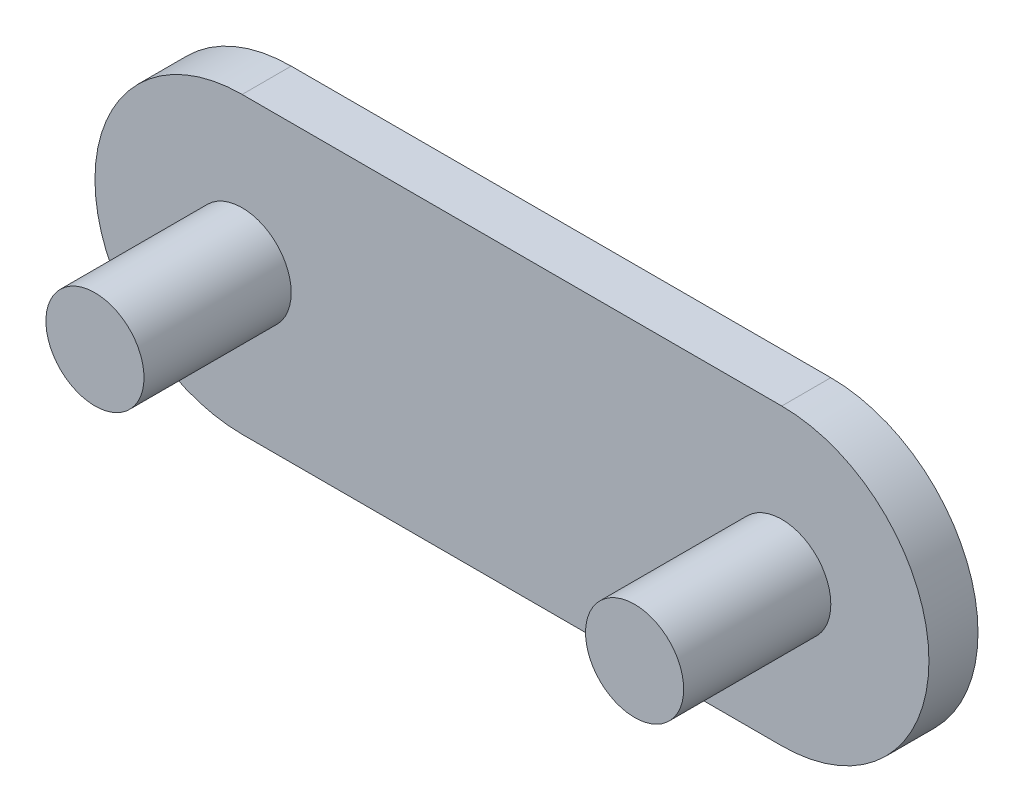
ISO-10303-21;
HEADER;
FILE_DESCRIPTION(('STEP AP214'),'2;1');
FILE_NAME('part.step','',(''),(''),'','','');
FILE_SCHEMA(('AUTOMOTIVE_DESIGN { 1 0 10303 214 1 1 1 1 }'));
ENDSEC;
DATA;
#1=APPLICATION_CONTEXT('core data for automotive mechanical design processes');
#2=APPLICATION_PROTOCOL_DEFINITION('international standard','automotive_design',2000,#1);
#3=PRODUCT_CONTEXT('',#1,'mechanical');
#4=PRODUCT('Part','Part','',(#3));
#5=PRODUCT_RELATED_PRODUCT_CATEGORY('part','',(#4));
#6=PRODUCT_DEFINITION_FORMATION('','',#4);
#7=PRODUCT_DEFINITION_CONTEXT('part definition',#1,'design');
#8=PRODUCT_DEFINITION('design','',#6,#7);
#9=PRODUCT_DEFINITION_SHAPE('','',#8);
#10=(LENGTH_UNIT() NAMED_UNIT(*) SI_UNIT(.MILLI.,.METRE.));
#11=(NAMED_UNIT(*) PLANE_ANGLE_UNIT() SI_UNIT($,.RADIAN.));
#12=(NAMED_UNIT(*) SI_UNIT($,.STERADIAN.) SOLID_ANGLE_UNIT());
#13=UNCERTAINTY_MEASURE_WITH_UNIT(LENGTH_MEASURE(1.E-05),#10,'distance_accuracy_value','');
#14=(GEOMETRIC_REPRESENTATION_CONTEXT(3) GLOBAL_UNCERTAINTY_ASSIGNED_CONTEXT((#13)) GLOBAL_UNIT_ASSIGNED_CONTEXT((#10,
#11,#12)) REPRESENTATION_CONTEXT('',''));
#15=CARTESIAN_POINT('',(0.,0.,0.));
#16=DIRECTION('',(0.,0.,1.));
#17=DIRECTION('',(1.,0.,0.));
#18=AXIS2_PLACEMENT_3D('',#15,#16,#17);
#19=CARTESIAN_POINT('',(27.5,0.,-5.));
#20=DIRECTION('',(0.,0.,1.));
#21=DIRECTION('',(1.,0.,0.));
#22=AXIS2_PLACEMENT_3D('',#19,#20,#21);
#23=CYLINDRICAL_SURFACE('',#22,15.);
#24=CARTESIAN_POINT('',(27.5,0.,0.));
#25=DIRECTION('',(0.,0.,1.));
#26=DIRECTION('',(1.,0.,0.));
#27=AXIS2_PLACEMENT_3D('',#24,#25,#26);
#28=CIRCLE('',#27,15.);
#29=CARTESIAN_POINT('',(27.5,-15.,0.));
#30=VERTEX_POINT('',#29);
#31=CARTESIAN_POINT('',(27.5,15.,0.));
#32=VERTEX_POINT('',#31);
#33=EDGE_CURVE('E110',#30,#32,#28,.T.);
#34=ORIENTED_EDGE('',*,*,#33,.F.);
#35=DIRECTION('',(0.,0.,1.));
#36=VECTOR('',#35,1.);
#37=CARTESIAN_POINT('',(27.5,-15.,-5.));
#38=LINE('',#37,#36);
#39=CARTESIAN_POINT('',(27.5,-15.,-5.));
#40=VERTEX_POINT('',#39);
#41=EDGE_CURVE('E11',#40,#30,#38,.T.);
#42=ORIENTED_EDGE('',*,*,#41,.F.);
#43=CARTESIAN_POINT('',(27.5,0.,-5.));
#44=DIRECTION('',(0.,0.,1.));
#45=DIRECTION('',(1.,0.,0.));
#46=AXIS2_PLACEMENT_3D('',#43,#44,#45);
#47=CIRCLE('',#46,15.);
#48=CARTESIAN_POINT('',(27.5,15.,-5.));
#49=VERTEX_POINT('',#48);
#50=EDGE_CURVE('E99',#40,#49,#47,.T.);
#51=ORIENTED_EDGE('',*,*,#50,.T.);
#52=DIRECTION('',(0.,0.,1.));
#53=VECTOR('',#52,1.);
#54=CARTESIAN_POINT('',(27.5,15.,-5.));
#55=LINE('',#54,#53);
#56=EDGE_CURVE('E42',#49,#32,#55,.T.);
#57=ORIENTED_EDGE('',*,*,#56,.T.);
#58=EDGE_LOOP('',(#34,#42,#51,#57));
#59=FACE_BOUND('',#58,.T.);
#60=ADVANCED_FACE('F41',(#59),#23,.T.);
#61=CARTESIAN_POINT('',(27.5,-15.,-5.));
#62=DIRECTION('',(0.,1.,0.));
#63=DIRECTION('',(-1.,0.,0.));
#64=AXIS2_PLACEMENT_3D('',#61,#62,#63);
#65=PLANE('',#64);
#66=DIRECTION('',(-1.,0.,0.));
#67=VECTOR('',#66,1.);
#68=CARTESIAN_POINT('',(27.5,-15.,0.));
#69=LINE('',#68,#67);
#70=CARTESIAN_POINT('',(-27.5,-15.,0.));
#71=VERTEX_POINT('',#70);
#72=EDGE_CURVE('E105',#30,#71,#69,.T.);
#73=ORIENTED_EDGE('',*,*,#72,.T.);
#74=DIRECTION('',(0.,0.,1.));
#75=VECTOR('',#74,1.);
#76=CARTESIAN_POINT('',(-27.5,-15.,-5.));
#77=LINE('',#76,#75);
#78=CARTESIAN_POINT('',(-27.5,-15.,-5.));
#79=VERTEX_POINT('',#78);
#80=EDGE_CURVE('E49',#79,#71,#77,.T.);
#81=ORIENTED_EDGE('',*,*,#80,.F.);
#82=DIRECTION('',(-1.,0.,0.));
#83=VECTOR('',#82,1.);
#84=CARTESIAN_POINT('',(27.5,-15.,-5.));
#85=LINE('',#84,#83);
#86=EDGE_CURVE('E100',#40,#79,#85,.T.);
#87=ORIENTED_EDGE('',*,*,#86,.F.);
#88=ORIENTED_EDGE('',*,*,#41,.T.);
#89=EDGE_LOOP('',(#73,#81,#87,#88));
#90=FACE_BOUND('',#89,.T.);
#91=ADVANCED_FACE('F113',(#90),#65,.F.);
#92=CARTESIAN_POINT('',(-27.5,0.,-5.));
#93=DIRECTION('',(0.,0.,1.));
#94=DIRECTION('',(1.,0.,0.));
#95=AXIS2_PLACEMENT_3D('',#92,#93,#94);
#96=CYLINDRICAL_SURFACE('',#95,15.);
#97=CARTESIAN_POINT('',(-27.5,0.,0.));
#98=DIRECTION('',(0.,0.,1.));
#99=DIRECTION('',(1.,0.,0.));
#100=AXIS2_PLACEMENT_3D('',#97,#98,#99);
#101=CIRCLE('',#100,15.);
#102=CARTESIAN_POINT('',(-27.5,15.,0.));
#103=VERTEX_POINT('',#102);
#104=EDGE_CURVE('E93',#103,#71,#101,.T.);
#105=ORIENTED_EDGE('',*,*,#104,.F.);
#106=DIRECTION('',(0.,0.,1.));
#107=VECTOR('',#106,1.);
#108=CARTESIAN_POINT('',(-27.5,15.,-5.));
#109=LINE('',#108,#107);
#110=CARTESIAN_POINT('',(-27.5,15.,-5.));
#111=VERTEX_POINT('',#110);
#112=EDGE_CURVE('E88',#111,#103,#109,.T.);
#113=ORIENTED_EDGE('',*,*,#112,.F.);
#114=CARTESIAN_POINT('',(-27.5,0.,-5.));
#115=DIRECTION('',(0.,0.,1.));
#116=DIRECTION('',(1.,0.,0.));
#117=AXIS2_PLACEMENT_3D('',#114,#115,#116);
#118=CIRCLE('',#117,15.);
#119=EDGE_CURVE('E90',#111,#79,#118,.T.);
#120=ORIENTED_EDGE('',*,*,#119,.T.);
#121=ORIENTED_EDGE('',*,*,#80,.T.);
#122=EDGE_LOOP('',(#105,#113,#120,#121));
#123=FACE_BOUND('',#122,.T.);
#124=ADVANCED_FACE('F86',(#123),#96,.T.);
#125=CARTESIAN_POINT('',(27.5,15.,-5.));
#126=DIRECTION('',(0.,1.,0.));
#127=DIRECTION('',(-1.,0.,0.));
#128=AXIS2_PLACEMENT_3D('',#125,#126,#127);
#129=PLANE('',#128);
#130=DIRECTION('',(-1.,0.,0.));
#131=VECTOR('',#130,1.);
#132=CARTESIAN_POINT('',(27.5,15.,0.));
#133=LINE('',#132,#131);
#134=EDGE_CURVE('E109',#32,#103,#133,.T.);
#135=ORIENTED_EDGE('',*,*,#134,.F.);
#136=ORIENTED_EDGE('',*,*,#56,.F.);
#137=DIRECTION('',(-1.,0.,0.));
#138=VECTOR('',#137,1.);
#139=CARTESIAN_POINT('',(27.5,15.,-5.));
#140=LINE('',#139,#138);
#141=EDGE_CURVE('E96',#49,#111,#140,.T.);
#142=ORIENTED_EDGE('',*,*,#141,.T.);
#143=ORIENTED_EDGE('',*,*,#112,.T.);
#144=EDGE_LOOP('',(#135,#136,#142,#143));
#145=FACE_BOUND('',#144,.T.);
#146=ADVANCED_FACE('F97',(#145),#129,.T.);
#147=CARTESIAN_POINT('',(27.5,0.,-5.));
#148=DIRECTION('',(0.,0.,1.));
#149=DIRECTION('',(1.,0.,0.));
#150=AXIS2_PLACEMENT_3D('',#147,#148,#149);
#151=PLANE('',#150);
#152=ORIENTED_EDGE('',*,*,#50,.F.);
#153=ORIENTED_EDGE('',*,*,#86,.T.);
#154=ORIENTED_EDGE('',*,*,#119,.F.);
#155=ORIENTED_EDGE('',*,*,#141,.F.);
#156=EDGE_LOOP('',(#152,#153,#154,#155));
#157=FACE_BOUND('',#156,.T.);
#158=ADVANCED_FACE('F92',(#157),#151,.F.);
#159=CARTESIAN_POINT('',(27.5,0.,0.));
#160=DIRECTION('',(0.,0.,1.));
#161=DIRECTION('',(1.,0.,0.));
#162=AXIS2_PLACEMENT_3D('',#159,#160,#161);
#163=PLANE('',#162);
#164=CARTESIAN_POINT('',(27.5,0.,0.));
#165=DIRECTION('',(0.,0.,1.));
#166=DIRECTION('',(1.,0.,0.));
#167=AXIS2_PLACEMENT_3D('',#164,#165,#166);
#168=CIRCLE('',#167,5.);
#169=CARTESIAN_POINT('',(32.5,0.,0.));
#170=VERTEX_POINT('',#169);
#171=EDGE_CURVE('E157',#170,#170,#168,.T.);
#172=ORIENTED_EDGE('',*,*,#171,.F.);
#173=EDGE_LOOP('',(#172));
#174=FACE_BOUND('',#173,.T.);
#175=CARTESIAN_POINT('',(-27.5,0.,0.));
#176=DIRECTION('',(0.,0.,1.));
#177=DIRECTION('',(1.,0.,0.));
#178=AXIS2_PLACEMENT_3D('',#175,#176,#177);
#179=CIRCLE('',#178,5.);
#180=CARTESIAN_POINT('',(-22.5,0.,0.));
#181=VERTEX_POINT('',#180);
#182=EDGE_CURVE('E158',#181,#181,#179,.T.);
#183=ORIENTED_EDGE('',*,*,#182,.F.);
#184=EDGE_LOOP('',(#183));
#185=FACE_BOUND('',#184,.T.);
#186=ORIENTED_EDGE('',*,*,#33,.T.);
#187=ORIENTED_EDGE('',*,*,#134,.T.);
#188=ORIENTED_EDGE('',*,*,#104,.T.);
#189=ORIENTED_EDGE('',*,*,#72,.F.);
#190=EDGE_LOOP('',(#186,#187,#188,#189));
#191=FACE_BOUND('',#190,.T.);
#192=ADVANCED_FACE('F116',(#174,#185,#191),#163,.T.);
#193=CARTESIAN_POINT('',(-27.5,0.,15.));
#194=DIRECTION('',(0.,0.,-1.));
#195=DIRECTION('',(-1.,0.,0.));
#196=AXIS2_PLACEMENT_3D('',#193,#194,#195);
#197=CYLINDRICAL_SURFACE('',#196,5.);
#198=CARTESIAN_POINT('',(-27.5,0.,15.));
#199=DIRECTION('',(0.,0.,1.));
#200=DIRECTION('',(1.,0.,0.));
#201=AXIS2_PLACEMENT_3D('',#198,#199,#200);
#202=CIRCLE('',#201,5.);
#203=CARTESIAN_POINT('',(-22.5,0.,15.));
#204=VERTEX_POINT('',#203);
#205=EDGE_CURVE('E112',#204,#204,#202,.T.);
#206=ORIENTED_EDGE('',*,*,#205,.F.);
#207=EDGE_LOOP('',(#206));
#208=FACE_BOUND('',#207,.T.);
#209=ORIENTED_EDGE('',*,*,#182,.T.);
#210=EDGE_LOOP('',(#209));
#211=FACE_BOUND('',#210,.T.);
#212=ADVANCED_FACE('F136',(#208,#211),#197,.T.);
#213=CARTESIAN_POINT('',(0.,0.,15.));
#214=DIRECTION('',(0.,0.,1.));
#215=DIRECTION('',(1.,0.,0.));
#216=AXIS2_PLACEMENT_3D('',#213,#214,#215);
#217=PLANE('',#216);
#218=ORIENTED_EDGE('',*,*,#205,.T.);
#219=EDGE_LOOP('',(#218));
#220=FACE_BOUND('',#219,.T.);
#221=ADVANCED_FACE('F143',(#220),#217,.T.);
#222=CARTESIAN_POINT('',(27.5,0.,15.));
#223=DIRECTION('',(0.,0.,-1.));
#224=DIRECTION('',(-1.,0.,0.));
#225=AXIS2_PLACEMENT_3D('',#222,#223,#224);
#226=CYLINDRICAL_SURFACE('',#225,5.);
#227=CARTESIAN_POINT('',(27.5,0.,15.));
#228=DIRECTION('',(0.,0.,1.));
#229=DIRECTION('',(1.,0.,0.));
#230=AXIS2_PLACEMENT_3D('',#227,#228,#229);
#231=CIRCLE('',#230,5.);
#232=CARTESIAN_POINT('',(32.5,0.,15.));
#233=VERTEX_POINT('',#232);
#234=EDGE_CURVE('E160',#233,#233,#231,.T.);
#235=ORIENTED_EDGE('',*,*,#234,.F.);
#236=EDGE_LOOP('',(#235));
#237=FACE_BOUND('',#236,.T.);
#238=ORIENTED_EDGE('',*,*,#171,.T.);
#239=EDGE_LOOP('',(#238));
#240=FACE_BOUND('',#239,.T.);
#241=ADVANCED_FACE('F144',(#237,#240),#226,.T.);
#242=CARTESIAN_POINT('',(0.,0.,15.));
#243=DIRECTION('',(0.,0.,1.));
#244=DIRECTION('',(1.,0.,0.));
#245=AXIS2_PLACEMENT_3D('',#242,#243,#244);
#246=PLANE('',#245);
#247=ORIENTED_EDGE('',*,*,#234,.T.);
#248=EDGE_LOOP('',(#247));
#249=FACE_BOUND('',#248,.T.);
#250=ADVANCED_FACE('F149',(#249),#246,.T.);
#251=CLOSED_SHELL('',(#60,#91,#124,#146,#158,#192,#212,#221,#241,#250));
#252=MANIFOLD_SOLID_BREP('B2',#251);
#253=ADVANCED_BREP_SHAPE_REPRESENTATION('',(#18,#252),#14);
#254=SHAPE_DEFINITION_REPRESENTATION(#9,#253);
ENDSEC;
END-ISO-10303-21;
